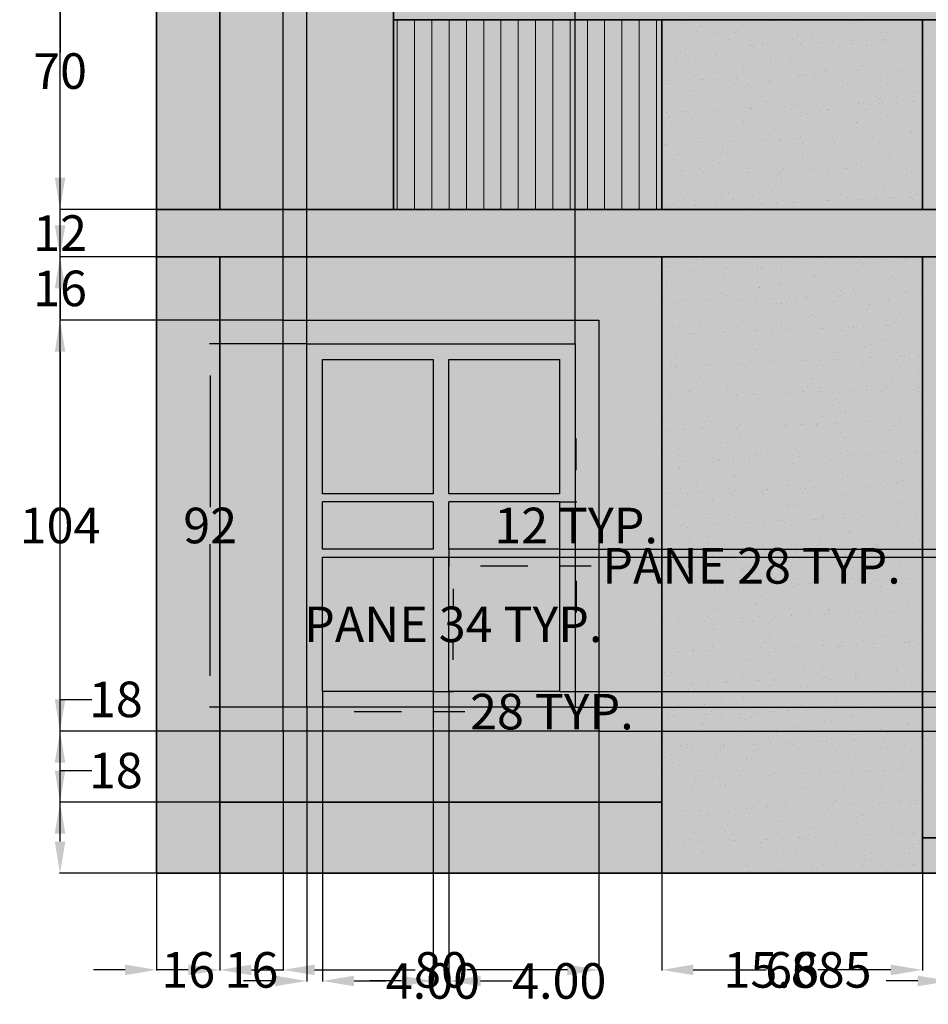
# Model space of a CAD drawing. Units: inches. Extents: x 207 to 609, y 30 to 576.
# Tile 1 of 4: x 215 to 445, y 30 to 279. Entities that reach past the tile are written whole.
import ezdxf

# ---------------------------------------------------------------- set-up
doc = ezdxf.new("R2010")
doc.units = ezdxf.units.IN
doc.header["$MEASUREMENT"] = 0
doc.layers.get('0').update_dxf_attribs({"color": 250})
for name, color, linetype, lineweight in [('A-ANNO-DIMS', 2, 'Continuous', 18), ('A-ELEV', 7, 'Continuous', 35), ('A-ELEV-PATT', 251, 'Continuous', 13), ('A-ELEV-PATT-CLAD', 67, 'Continuous', 13), ('A-ELEV-PATT-WOOD', 19, 'Continuous', 13), ('A-GLAZ', 4, 'Continuous', 25)]:
    doc.layers.add(name, color=color, linetype=linetype, lineweight=lineweight)
doc.styles.get("Standard").update_dxf_attribs({"font": 'arial.ttf'})
doc.dimstyles.get("Standard").update_dxf_attribs({"dimtxt": 9, "dimasz": 8, "dimexe": 0.18, "dimexo": 0.0625, "dimgap": 0.09, "dimtad": 0, "dimtih": 1, "dimtoh": 1, "dimdec": 0, "dimzin": 0, "dimdsep": 46, "dimlunit": 3, "dimtxsty": 'Standard', "dimcen": 0.09, "dimadec": 0, "dimazin": 0, "dimtfac": 1, "dimtdec": 0, "dimtofl": 0, "dimtmove": 0, "dimatfit": 3, "dimfxl": 1, "dimtolj": 1, "dimtzin": 0, "dimarcsym": 0})

# ---------------------------------------------------------------- blocks, each defined once
blk = doc.blocks.new('WIN-PANE-LG')
for p, q in [((0, 34), (28, 34)), ((0, 0), (0, 34)), ((28, 34), (28, 0)), ((28, 0), (0, 0))]:
    blk.add_line(p, q)
blk = doc.blocks.new('WIN-PANE-SM')
for p, q in [((28, 12), (0, 12)), ((0, 0), (0, 12)), ((28, 12), (28, 0)), ((28, 0), (0, 0))]:
    blk.add_line(p, q)
blk = doc.blocks.new('*D3')
at = {"layer": 'A-ANNO-DIMS', "color": 0, "lineweight": -2, "transparency": 16777216}
for p, q in [((319.76, 142.79), (324.98, 142.79)), ((324.8, 134.79), (324.8, 130.47)), ((324.8, 116.79), (324.8, 121.1)), ((319.76, 108.79), (324.98, 108.79))]:
    blk.add_line(p, q, dxfattribs=at)
at = {"layer": 'A-ANNO-DIMS', "color": 0, "transparency": 16777216}
for points in [[(323.46, 134.79), (326.13, 134.79), (324.8, 142.79)], [(323.46, 116.79), (326.13, 116.79), (324.8, 108.79)]]:
    blk.add_solid(points, dxfattribs=at)
at = {"layer": 'Defpoints', "color": 0, "transparency": 16777216}
for p in [(319.7, 142.79), (324.8, 142.79), (319.7, 108.79)]:
    blk.add_point(p, dxfattribs=at)
at = {"layer": 'A-ANNO-DIMS', "color": 0, "transparency": 16777216, "insert": (324.8, 125.79), "char_height": 9, "attachment_point": 5}
blk.add_mtext('\\A1;PANE 34 TYP.', dxfattribs=at)
blk = doc.blocks.new('*D4')
at = {"layer": 'A-ANNO-DIMS', "color": 0, "lineweight": -2, "transparency": 16777216}
for p, q in [((291.7, 108.72), (291.7, 103.51)), ((319.7, 108.72), (319.7, 103.51)), ((299.7, 103.69), (311.7, 103.69)), ((319.7, 103.69), (327.7, 103.69))]:
    blk.add_line(p, q, dxfattribs=at)
at = {"layer": 'A-ANNO-DIMS', "color": 0, "transparency": 16777216}
for points in [[(299.7, 105.02), (299.7, 102.35), (291.7, 103.69)], [(311.7, 105.02), (311.7, 102.35), (319.7, 103.69)]]:
    blk.add_solid(points, dxfattribs=at)
at = {"layer": 'Defpoints', "color": 0, "transparency": 16777216}
for p in [(291.7, 108.79), (319.7, 108.79), (319.7, 103.69)]:
    blk.add_point(p, dxfattribs=at)
at = {"layer": 'A-ANNO-DIMS', "color": 0, "transparency": 16777216, "insert": (349.77, 103.69), "char_height": 9, "attachment_point": 5}
blk.add_mtext('\\A1;28 TYP.', dxfattribs=at)
blk = doc.blocks.new('*D5')
at = {"layer": 'A-ANNO-DIMS', "color": 0, "lineweight": -2, "transparency": 16777216}
for p, q in [((323.7, 144.72), (323.7, 140.41)), ((351.7, 144.72), (351.7, 140.41)), ((331.7, 140.59), (343.7, 140.59)), ((351.7, 140.59), (359.7, 140.59))]:
    blk.add_line(p, q, dxfattribs=at)
at = {"layer": 'A-ANNO-DIMS', "color": 0, "transparency": 16777216}
for points in [[(331.7, 141.92), (331.7, 139.25), (323.7, 140.59)], [(343.7, 141.92), (343.7, 139.25), (351.7, 140.59)]]:
    blk.add_solid(points, dxfattribs=at)
at = {"layer": 'Defpoints', "color": 0, "transparency": 16777216}
for p in [(323.7, 144.79), (351.7, 144.79), (351.7, 140.59)]:
    blk.add_point(p, dxfattribs=at)
at = {"layer": 'A-ANNO-DIMS', "color": 0, "transparency": 16777216, "insert": (400.33, 140.59), "char_height": 9, "attachment_point": 5}
blk.add_mtext('\\A1;PANE 28 TYP.', dxfattribs=at)
blk = doc.blocks.new('*D6')
at = {"layer": 'A-ANNO-DIMS', "color": 0, "lineweight": -2, "transparency": 16777216}
for p, q in [((355.9, 164.79), (355.9, 172.79)), ((351.76, 156.79), (356.08, 156.79)), ((351.76, 144.79), (356.08, 144.79)), ((355.9, 136.79), (355.9, 128.79))]:
    blk.add_line(p, q, dxfattribs=at)
at = {"layer": 'A-ANNO-DIMS', "color": 0, "transparency": 16777216}
for points in [[(354.56, 164.79), (357.23, 164.79), (355.9, 156.79)], [(354.56, 136.79), (357.23, 136.79), (355.9, 144.79)]]:
    blk.add_solid(points, dxfattribs=at)
at = {"layer": 'Defpoints', "color": 0, "transparency": 16777216}
for p in [(351.7, 156.79), (355.9, 156.79), (351.7, 144.79)]:
    blk.add_point(p, dxfattribs=at)
at = {"layer": 'A-ANNO-DIMS', "color": 0, "transparency": 16777216, "insert": (355.9, 150.79), "char_height": 9, "attachment_point": 5}
blk.add_mtext('\\A1;12 TYP.', dxfattribs=at)
blk = doc.blocks.new('*D8')
at = {"layer": 'A-ANNO-DIMS', "color": 0, "lineweight": -2, "transparency": 16777216}
for p, q in [((249.63, 542.79), (225.07, 542.79)), ((225.25, 534.79), (225.25, 307.47)), ((225.25, 70.79), (225.25, 298.1)), ((249.63, 62.79), (225.07, 62.79))]:
    blk.add_line(p, q, dxfattribs=at)
at = {"layer": 'A-ANNO-DIMS', "color": 0, "transparency": 16777216}
for points in [[(223.91, 534.79), (226.58, 534.79), (225.25, 542.79)], [(223.91, 70.79), (226.58, 70.79), (225.25, 62.79)]]:
    blk.add_solid(points, dxfattribs=at)
at = {"layer": 'Defpoints', "color": 0, "transparency": 16777216}
for p in [(225.25, 542.79), (249.7, 542.79), (249.7, 62.79)]:
    blk.add_point(p, dxfattribs=at)
at = {"layer": 'A-ANNO-DIMS', "color": 0, "transparency": 16777216, "insert": (225.25, 302.79), "char_height": 9, "attachment_point": 5}
blk.add_mtext('\\A1;480', dxfattribs=at)
blk = doc.blocks.new('*D10')
at = {"layer": 'A-ANNO-DIMS', "color": 0, "lineweight": -2, "transparency": 16777216}
for p, q in [((225.25, 80.79), (225.25, 88.79)), ((225.25, 88.79), (233.25, 88.79)), ((265.63, 80.79), (225.07, 80.79)), ((225.25, 70.79), (225.25, 72.79)), ((265.63, 62.79), (225.07, 62.79))]:
    blk.add_line(p, q, dxfattribs=at)
at = {"layer": 'A-ANNO-DIMS', "color": 0, "transparency": 16777216}
for points in [[(223.91, 72.79), (226.58, 72.79), (225.25, 80.79)], [(223.91, 70.79), (226.58, 70.79), (225.25, 62.79)]]:
    blk.add_solid(points, dxfattribs=at)
at = {"layer": 'Defpoints', "color": 0, "transparency": 16777216}
for p in [(225.25, 80.79), (265.7, 80.79), (265.7, 62.79)]:
    blk.add_point(p, dxfattribs=at)
at = {"layer": 'A-ANNO-DIMS', "color": 0, "transparency": 16777216, "insert": (239.37, 88.79), "char_height": 9, "attachment_point": 5}
blk.add_mtext('\\A1;18', dxfattribs=at)
blk = doc.blocks.new('*D11')
at = {"layer": 'A-ANNO-DIMS', "color": 0, "lineweight": -2, "transparency": 16777216}
for p, q in [((225.25, 98.79), (225.25, 106.79)), ((225.25, 106.79), (233.25, 106.79)), ((281.63, 98.79), (225.07, 98.79)), ((225.25, 88.79), (225.25, 90.79)), ((265.63, 80.79), (225.07, 80.79))]:
    blk.add_line(p, q, dxfattribs=at)
at = {"layer": 'A-ANNO-DIMS', "color": 0, "transparency": 16777216}
for points in [[(223.91, 90.79), (226.58, 90.79), (225.25, 98.79)], [(223.91, 88.79), (226.58, 88.79), (225.25, 80.79)]]:
    blk.add_solid(points, dxfattribs=at)
at = {"layer": 'Defpoints', "color": 0, "transparency": 16777216}
for p in [(225.25, 98.79), (281.7, 98.79), (265.7, 80.79)]:
    blk.add_point(p, dxfattribs=at)
at = {"layer": 'A-ANNO-DIMS', "color": 0, "transparency": 16777216, "insert": (239.37, 106.79), "char_height": 9, "attachment_point": 5}
blk.add_mtext('\\A1;18', dxfattribs=at)
blk = doc.blocks.new('*D12')
at = {"layer": 'A-ANNO-DIMS', "color": 0, "lineweight": -2, "transparency": 16777216}
for p, q in [((281.63, 202.79), (225.07, 202.79)), ((225.25, 194.79), (225.25, 155.47)), ((225.25, 106.79), (225.25, 146.1)), ((281.63, 98.79), (225.07, 98.79))]:
    blk.add_line(p, q, dxfattribs=at)
at = {"layer": 'A-ANNO-DIMS', "color": 0, "transparency": 16777216}
for points in [[(223.91, 194.79), (226.58, 194.79), (225.25, 202.79)], [(223.91, 106.79), (226.58, 106.79), (225.25, 98.79)]]:
    blk.add_solid(points, dxfattribs=at)
at = {"layer": 'Defpoints', "color": 0, "transparency": 16777216}
for p in [(225.25, 202.79), (281.7, 202.79), (281.7, 98.79)]:
    blk.add_point(p, dxfattribs=at)
at = {"layer": 'A-ANNO-DIMS', "color": 0, "transparency": 16777216, "insert": (225.25, 150.79), "char_height": 9, "attachment_point": 5}
blk.add_mtext('\\A1;104', dxfattribs=at)
blk = doc.blocks.new('*D13')
at = {"layer": 'A-ANNO-DIMS', "color": 0, "lineweight": -2, "transparency": 16777216}
for p, q in [((225.25, 226.79), (225.25, 234.79)), ((265.63, 218.79), (225.07, 218.79)), ((281.63, 202.79), (225.07, 202.79)), ((225.25, 194.79), (225.25, 186.79))]:
    blk.add_line(p, q, dxfattribs=at)
at = {"layer": 'A-ANNO-DIMS', "color": 0, "transparency": 16777216}
for points in [[(223.91, 226.79), (226.58, 226.79), (225.25, 218.79)], [(223.91, 194.79), (226.58, 194.79), (225.25, 202.79)]]:
    blk.add_solid(points, dxfattribs=at)
at = {"layer": 'Defpoints', "color": 0, "transparency": 16777216}
for p in [(225.25, 218.79), (265.7, 218.79), (281.7, 202.79)]:
    blk.add_point(p, dxfattribs=at)
at = {"layer": 'A-ANNO-DIMS', "color": 0, "transparency": 16777216, "insert": (225.25, 210.79), "char_height": 9, "attachment_point": 5}
blk.add_mtext('\\A1;16', dxfattribs=at)
blk = doc.blocks.new('*D14')
at = {"layer": 'A-ANNO-DIMS', "color": 0, "lineweight": -2, "transparency": 16777216}
for p, q in [((225.25, 238.79), (225.25, 246.79)), ((265.63, 230.79), (225.07, 230.79)), ((265.63, 218.79), (225.07, 218.79)), ((225.25, 210.79), (225.25, 202.79))]:
    blk.add_line(p, q, dxfattribs=at)
at = {"layer": 'A-ANNO-DIMS', "color": 0, "transparency": 16777216}
for points in [[(223.91, 238.79), (226.58, 238.79), (225.25, 230.79)], [(223.91, 210.79), (226.58, 210.79), (225.25, 218.79)]]:
    blk.add_solid(points, dxfattribs=at)
at = {"layer": 'Defpoints', "color": 0, "transparency": 16777216}
for p in [(225.25, 230.79), (265.7, 230.79), (265.7, 218.79)]:
    blk.add_point(p, dxfattribs=at)
at = {"layer": 'A-ANNO-DIMS', "color": 0, "transparency": 16777216, "insert": (225.25, 224.79), "char_height": 9, "attachment_point": 5}
blk.add_mtext('\\A1;12', dxfattribs=at)
blk = doc.blocks.new('*D15')
at = {"layer": 'A-ANNO-DIMS', "color": 0, "lineweight": -2, "transparency": 16777216}
for p, q in [((265.63, 300.79), (225.07, 300.79)), ((225.25, 292.79), (225.25, 270.47)), ((225.25, 238.79), (225.25, 261.1)), ((265.63, 230.79), (225.07, 230.79))]:
    blk.add_line(p, q, dxfattribs=at)
at = {"layer": 'A-ANNO-DIMS', "color": 0, "transparency": 16777216}
for points in [[(223.91, 292.79), (226.58, 292.79), (225.25, 300.79)], [(223.91, 238.79), (226.58, 238.79), (225.25, 230.79)]]:
    blk.add_solid(points, dxfattribs=at)
at = {"layer": 'Defpoints', "color": 0, "transparency": 16777216}
for p in [(225.25, 300.79), (265.7, 300.79), (265.7, 230.79)]:
    blk.add_point(p, dxfattribs=at)
at = {"layer": 'A-ANNO-DIMS', "color": 0, "transparency": 16777216, "insert": (225.25, 265.79), "char_height": 9, "attachment_point": 5}
blk.add_mtext('\\A1;70', dxfattribs=at)
blk = doc.blocks.new('*D27')
at = {"layer": 'A-ANNO-DIMS', "color": 0, "lineweight": -2, "transparency": 16777216}
for p, q in [((249.7, 62.72), (249.7, 38.16)), ((265.7, 62.72), (265.7, 38.16)), ((241.7, 38.34), (233.7, 38.34)), ((273.7, 38.34), (281.7, 38.34))]:
    blk.add_line(p, q, dxfattribs=at)
at = {"layer": 'A-ANNO-DIMS', "color": 0, "transparency": 16777216}
for points in [[(241.7, 39.67), (241.7, 37), (249.7, 38.34)], [(273.7, 39.67), (273.7, 37), (265.7, 38.34)]]:
    blk.add_solid(points, dxfattribs=at)
at = {"layer": 'Defpoints', "color": 0, "transparency": 16777216}
for p in [(249.7, 62.79), (265.7, 62.79), (265.7, 38.34)]:
    blk.add_point(p, dxfattribs=at)
at = {"layer": 'A-ANNO-DIMS', "color": 0, "transparency": 16777216, "insert": (257.7, 38.34), "char_height": 9, "attachment_point": 5}
blk.add_mtext('\\A1;16', dxfattribs=at)
blk = doc.blocks.new('*D28')
at = {"layer": 'A-ANNO-DIMS', "color": 0, "lineweight": -2, "transparency": 16777216}
for p, q in [((281.7, 98.72), (281.7, 38.16)), ((265.7, 62.72), (265.7, 38.16)), ((257.7, 38.34), (249.7, 38.34)), ((289.7, 38.34), (297.7, 38.34))]:
    blk.add_line(p, q, dxfattribs=at)
at = {"layer": 'A-ANNO-DIMS', "color": 0, "transparency": 16777216}
for points in [[(257.7, 39.67), (257.7, 37), (265.7, 38.34)], [(289.7, 39.67), (289.7, 37), (281.7, 38.34)]]:
    blk.add_solid(points, dxfattribs=at)
at = {"layer": 'Defpoints', "color": 0, "transparency": 16777216}
for p in [(281.7, 98.79), (265.7, 62.79), (281.7, 38.34)]:
    blk.add_point(p, dxfattribs=at)
at = {"layer": 'A-ANNO-DIMS', "color": 0, "transparency": 16777216, "insert": (273.7, 38.34), "char_height": 9, "attachment_point": 5}
blk.add_mtext('\\A1;16', dxfattribs=at)
blk = doc.blocks.new('*D29')
at = {"layer": 'A-ANNO-DIMS', "color": 0, "lineweight": -2, "transparency": 16777216}
for p, q in [((281.7, 98.72), (281.7, 38.16)), ((361.7, 98.72), (361.7, 38.16)), ((289.7, 38.34), (315.17, 38.34)), ((353.7, 38.34), (328.22, 38.34))]:
    blk.add_line(p, q, dxfattribs=at)
at = {"layer": 'A-ANNO-DIMS', "color": 0, "transparency": 16777216}
for points in [[(289.7, 39.67), (289.7, 37), (281.7, 38.34)], [(353.7, 39.67), (353.7, 37), (361.7, 38.34)]]:
    blk.add_solid(points, dxfattribs=at)
at = {"layer": 'Defpoints', "color": 0, "transparency": 16777216}
for p in [(281.7, 98.79), (361.7, 98.79), (361.7, 38.34)]:
    blk.add_point(p, dxfattribs=at)
at = {"layer": 'A-ANNO-DIMS', "color": 0, "transparency": 16777216, "insert": (321.7, 38.34), "char_height": 9, "attachment_point": 5}
blk.add_mtext('\\A1;80', dxfattribs=at)
blk = doc.blocks.new('*D30')
at = {"layer": 'A-ANNO-DIMS', "color": 0, "lineweight": -2, "transparency": 16777216}
for p, q in [((361.7, 98.72), (361.7, 38.16)), ((377.58, 62.72), (377.58, 38.16)), ((353.7, 38.34), (345.7, 38.34)), ((385.58, 38.34), (393.58, 38.34))]:
    blk.add_line(p, q, dxfattribs=at)
at = {"layer": 'A-ANNO-DIMS', "color": 0, "transparency": 16777216}
for points in [[(353.7, 39.67), (353.7, 37), (361.7, 38.34)], [(385.58, 39.67), (385.58, 37), (377.58, 38.34)]]:
    blk.add_solid(points, dxfattribs=at)
at = {"layer": 'Defpoints', "color": 0, "transparency": 16777216}
for p in [(361.7, 98.79), (377.58, 62.79), (377.58, 38.34)]:
    blk.add_point(p, dxfattribs=at)
at = {"layer": 'A-ANNO-DIMS', "color": 0, "transparency": 16777216, "insert": (411.96, 38.34), "char_height": 9, "attachment_point": 5}
blk.add_mtext('\\A1;15.885', dxfattribs=at)
blk = doc.blocks.new('*D31')
at = {"layer": 'A-ANNO-DIMS', "color": 0, "lineweight": -2, "transparency": 16777216}
for p, q in [((377.58, 62.72), (377.58, 38.16)), ((443.58, 62.72), (443.58, 38.16)), ((385.58, 38.34), (404.02, 38.34)), ((435.58, 38.34), (417.14, 38.34))]:
    blk.add_line(p, q, dxfattribs=at)
at = {"layer": 'A-ANNO-DIMS', "color": 0, "transparency": 16777216}
for points in [[(385.58, 39.67), (385.58, 37), (377.58, 38.34)], [(435.58, 39.67), (435.58, 37), (443.58, 38.34)]]:
    blk.add_solid(points, dxfattribs=at)
at = {"layer": 'Defpoints', "color": 0, "transparency": 16777216}
for p in [(377.58, 62.79), (443.58, 62.79), (443.58, 38.34)]:
    blk.add_point(p, dxfattribs=at)
at = {"layer": 'A-ANNO-DIMS', "color": 0, "transparency": 16777216, "insert": (410.58, 38.34), "char_height": 9, "attachment_point": 5}
blk.add_mtext('\\A1;66', dxfattribs=at)
blk = doc.blocks.new('*D32')
at = {"layer": 'A-ANNO-DIMS', "color": 0, "lineweight": -2, "transparency": 16777216}
for p, q in [((450.42, 269.6), (450.42, 38.16)), ((443.58, 62.72), (443.58, 38.16)), ((435.58, 38.34), (427.58, 38.34)), ((458.42, 38.34), (466.42, 38.34))]:
    blk.add_line(p, q, dxfattribs=at)
at = {"layer": 'A-ANNO-DIMS', "color": 0, "transparency": 16777216}
for points in [[(435.58, 39.67), (435.58, 37), (443.58, 38.34)], [(458.42, 39.67), (458.42, 37), (450.42, 38.34)]]:
    blk.add_solid(points, dxfattribs=at)
at = {"layer": 'Defpoints', "color": 0, "transparency": 16777216}
for p in [(450.42, 269.66), (443.58, 62.79), (450.42, 38.34)]:
    blk.add_point(p, dxfattribs=at)
at = {"layer": 'A-ANNO-DIMS', "color": 0, "transparency": 16777216, "insert": (481.71, 38.34), "char_height": 9, "attachment_point": 5}
blk.add_mtext('\\A1;6.844', dxfattribs=at)
blk = doc.blocks.new('*D61')
at = {"layer": 'A-ANNO-DIMS', "color": 0, "lineweight": -2, "transparency": 16777216}
for p, q in [((287.63, 196.79), (263.07, 196.79)), ((263.25, 188.79), (263.25, 155.47)), ((263.25, 112.79), (263.25, 146.1)), ((287.63, 104.79), (263.07, 104.79))]:
    blk.add_line(p, q, dxfattribs=at)
at = {"layer": 'A-ANNO-DIMS', "color": 0, "transparency": 16777216}
for points in [[(261.91, 188.79), (264.58, 188.79), (263.25, 196.79)], [(261.91, 112.79), (264.58, 112.79), (263.25, 104.79)]]:
    blk.add_solid(points, dxfattribs=at)
at = {"layer": 'Defpoints', "color": 0, "transparency": 16777216}
for p in [(263.25, 196.79), (287.7, 196.79), (287.7, 104.79)]:
    blk.add_point(p, dxfattribs=at)
at = {"layer": 'A-ANNO-DIMS', "color": 0, "transparency": 16777216, "insert": (263.25, 150.79), "char_height": 9, "attachment_point": 5}
blk.add_mtext('\\A1;92', dxfattribs=at)
blk = doc.blocks.new('*D71')
at = {"layer": 'A-ANNO-DIMS', "color": 0, "lineweight": -2, "transparency": 16777216}
for p, q in [((273.7, 570.04), (265.7, 570.04)), ((281.7, 202.85), (281.7, 570.22)), ((287.7, 196.85), (287.7, 570.22)), ((295.7, 570.04), (303.7, 570.04))]:
    blk.add_line(p, q, dxfattribs=at)
at = {"layer": 'A-ANNO-DIMS', "color": 0, "transparency": 16777216}
for points in [[(273.7, 571.37), (273.7, 568.7), (281.7, 570.04)], [(295.7, 571.37), (295.7, 568.7), (287.7, 570.04)]]:
    blk.add_solid(points, dxfattribs=at)
at = {"layer": 'Defpoints', "color": 0, "transparency": 16777216}
for p in [(287.7, 570.04), (281.7, 202.79), (287.7, 196.79)]:
    blk.add_point(p, dxfattribs=at)
at = {"layer": 'A-ANNO-DIMS', "color": 0, "transparency": 16777216, "insert": (315.48, 570.04), "char_height": 9, "attachment_point": 5}
blk.add_mtext('\\A1;6.00', dxfattribs=at)
blk = doc.blocks.new('*D72')
at = {"layer": 'A-ANNO-DIMS', "color": 0, "lineweight": -2, "transparency": 16777216}
for p, q in [((287.7, 196.85), (287.7, 570.22)), ((295.7, 570.04), (306.41, 570.04)), ((347.7, 570.04), (336.98, 570.04)), ((355.7, 196.85), (355.7, 570.22))]:
    blk.add_line(p, q, dxfattribs=at)
at = {"layer": 'A-ANNO-DIMS', "color": 0, "transparency": 16777216}
for points in [[(295.7, 571.37), (295.7, 568.7), (287.7, 570.04)], [(347.7, 571.37), (347.7, 568.7), (355.7, 570.04)]]:
    blk.add_solid(points, dxfattribs=at)
at = {"layer": 'Defpoints', "color": 0, "transparency": 16777216}
for p in [(355.7, 570.04), (287.7, 196.79), (355.7, 196.79)]:
    blk.add_point(p, dxfattribs=at)
at = {"layer": 'A-ANNO-DIMS', "color": 0, "transparency": 16777216, "insert": (321.7, 570.04), "char_height": 9, "attachment_point": 5}
blk.add_mtext('\\A1;68.00', dxfattribs=at)
blk = doc.blocks.new('*D73')
at = {"layer": 'A-ANNO-DIMS', "color": 0, "lineweight": -2, "transparency": 16777216}
for p, q in [((291.7, 108.72), (291.7, 35.36)), ((287.7, 104.72), (287.7, 35.36)), ((279.7, 35.54), (271.7, 35.54)), ((299.7, 35.54), (307.7, 35.54))]:
    blk.add_line(p, q, dxfattribs=at)
at = {"layer": 'A-ANNO-DIMS', "color": 0, "transparency": 16777216}
for points in [[(279.7, 36.87), (279.7, 34.2), (287.7, 35.54)], [(299.7, 36.87), (299.7, 34.2), (291.7, 35.54)]]:
    blk.add_solid(points, dxfattribs=at)
at = {"layer": 'Defpoints', "color": 0, "transparency": 16777216}
for p in [(291.7, 108.79), (287.7, 104.79), (291.7, 35.54)]:
    blk.add_point(p, dxfattribs=at)
at = {"layer": 'A-ANNO-DIMS', "color": 0, "transparency": 16777216, "insert": (319.64, 35.54), "char_height": 9, "attachment_point": 5}
blk.add_mtext('\\A1;4.00', dxfattribs=at)
blk = doc.blocks.new('*D74')
at = {"layer": 'A-ANNO-DIMS', "color": 0, "lineweight": -2, "transparency": 16777216}
for p, q in [((319.7, 108.72), (319.7, 35.36)), ((323.7, 108.72), (323.7, 35.36)), ((311.7, 35.54), (303.7, 35.54)), ((331.7, 35.54), (339.7, 35.54))]:
    blk.add_line(p, q, dxfattribs=at)
at = {"layer": 'A-ANNO-DIMS', "color": 0, "transparency": 16777216}
for points in [[(311.7, 36.87), (311.7, 34.2), (319.7, 35.54)], [(331.7, 36.87), (331.7, 34.2), (323.7, 35.54)]]:
    blk.add_solid(points, dxfattribs=at)
at = {"layer": 'Defpoints', "color": 0, "transparency": 16777216}
for p in [(319.7, 108.79), (323.7, 108.79), (323.7, 35.54)]:
    blk.add_point(p, dxfattribs=at)
at = {"layer": 'A-ANNO-DIMS', "color": 0, "transparency": 16777216, "insert": (351.64, 35.54), "char_height": 9, "attachment_point": 5}
blk.add_mtext('\\A1;4.00', dxfattribs=at)
blk = doc.blocks.new('*D75')
at = {"layer": 'A-ANNO-DIMS', "color": 0, "lineweight": -2, "transparency": 16777216}
for p, q in [((576.95, 112.79), (576.95, 120.79)), ((576.95, 120.79), (584.95, 120.79)), ((355.76, 104.79), (577.13, 104.79)), ((361.76, 98.79), (577.13, 98.79)), ((576.95, 90.79), (576.95, 82.79))]:
    blk.add_line(p, q, dxfattribs=at)
at = {"layer": 'A-ANNO-DIMS', "color": 0, "transparency": 16777216}
for points in [[(575.61, 112.79), (578.28, 112.79), (576.95, 104.79)], [(575.61, 90.79), (578.28, 90.79), (576.95, 98.79)]]:
    blk.add_solid(points, dxfattribs=at)
at = {"layer": 'Defpoints', "color": 0, "transparency": 16777216}
for p in [(355.7, 104.79), (576.95, 104.79), (361.7, 98.79)]:
    blk.add_point(p, dxfattribs=at)
at = {"layer": 'A-ANNO-DIMS', "color": 0, "transparency": 16777216, "insert": (596.73, 120.79), "char_height": 9, "attachment_point": 5}
blk.add_mtext('\\A1;6.00', dxfattribs=at)
blk = doc.blocks.new('*D76')
at = {"layer": 'A-ANNO-DIMS', "color": 0, "lineweight": -2, "transparency": 16777216}
for p, q in [((576.95, 116.79), (576.95, 124.79)), ((576.95, 124.79), (584.95, 124.79)), ((351.76, 108.79), (577.13, 108.79)), ((355.76, 104.79), (577.13, 104.79)), ((576.95, 96.79), (576.95, 88.79))]:
    blk.add_line(p, q, dxfattribs=at)
at = {"layer": 'A-ANNO-DIMS', "color": 0, "transparency": 16777216}
for points in [[(575.61, 116.79), (578.28, 116.79), (576.95, 108.79)], [(575.61, 96.79), (578.28, 96.79), (576.95, 104.79)]]:
    blk.add_solid(points, dxfattribs=at)
at = {"layer": 'Defpoints', "color": 0, "transparency": 16777216}
for p in [(351.7, 108.79), (576.95, 108.79), (355.7, 104.79)]:
    blk.add_point(p, dxfattribs=at)
at = {"layer": 'A-ANNO-DIMS', "color": 0, "transparency": 16777216, "insert": (596.89, 124.79), "char_height": 9, "attachment_point": 5}
blk.add_mtext('\\A1;4.00', dxfattribs=at)
blk = doc.blocks.new('*D77')
at = {"layer": 'A-ANNO-DIMS', "color": 0, "lineweight": -2, "transparency": 16777216}
for p, q in [((576.95, 152.79), (576.95, 160.79)), ((576.95, 160.79), (584.95, 160.79)), ((351.76, 144.79), (577.13, 144.79)), ((351.76, 142.79), (577.13, 142.79)), ((576.95, 134.79), (576.95, 126.79))]:
    blk.add_line(p, q, dxfattribs=at)
at = {"layer": 'A-ANNO-DIMS', "color": 0, "transparency": 16777216}
for points in [[(575.61, 152.79), (578.28, 152.79), (576.95, 144.79)], [(575.61, 134.79), (578.28, 134.79), (576.95, 142.79)]]:
    blk.add_solid(points, dxfattribs=at)
at = {"layer": 'Defpoints', "color": 0, "transparency": 16777216}
for p in [(351.7, 144.79), (576.95, 144.79), (351.7, 142.79)]:
    blk.add_point(p, dxfattribs=at)
at = {"layer": 'A-ANNO-DIMS', "color": 0, "transparency": 16777216, "insert": (596.79, 160.79), "char_height": 9, "attachment_point": 5}
blk.add_mtext('\\A1;2.00', dxfattribs=at)
blk = doc.blocks.new('*D79')
at = {"layer": 'A-ANNO-DIMS', "color": 0, "lineweight": -2, "transparency": 16777216}
for p, q in [((453.42, 240.19), (453.42, 35.36)), ((450.42, 237.19), (450.42, 35.36)), ((442.42, 35.54), (434.42, 35.54)), ((461.42, 35.54), (469.42, 35.54))]:
    blk.add_line(p, q, dxfattribs=at)
at = {"layer": 'A-ANNO-DIMS', "color": 0, "transparency": 16777216}
for points in [[(442.42, 36.87), (442.42, 34.2), (450.42, 35.54)], [(461.42, 36.87), (461.42, 34.2), (453.42, 35.54)]]:
    blk.add_solid(points, dxfattribs=at)
at = {"layer": 'Defpoints', "color": 0, "transparency": 16777216}
for p in [(453.42, 240.26), (450.42, 237.26), (453.42, 35.54)]:
    blk.add_point(p, dxfattribs=at)
at = {"layer": 'A-ANNO-DIMS', "color": 0, "transparency": 16777216, "insert": (481.19, 35.54), "char_height": 9, "attachment_point": 5}
blk.add_mtext('\\A1;3.00', dxfattribs=at)

msp = doc.modelspace()

# ---------------------------------------------------------------- hatches: boundary and pattern name
at = {"layer": 'A-ELEV-PATT'}
h = msp.add_hatch(color=256, dxfattribs=at)
h.dxf.hatch_style = 1
h.paths.add_polyline_path([(549.6956, 542.7864), (443.656, 542.7864), (443.656, 470.7864), (549.6956, 470.7864)])
h.paths.add_polyline_path([(549.6956, 230.7864), (249.6956, 230.7864), (249.6956, 218.7864), (549.6956, 218.7864)])
h.paths.add_polyline_path([(377.5808, 80.7864), (265.6956, 80.7864), (265.6956, 62.7864), (377.5808, 62.7864)])
h.paths.add_polyline_path([(549.6956, 71.7864), (443.5808, 71.7864), (443.5808, 62.7864), (549.6956, 62.7864)])
h = msp.add_hatch(color=256, dxfattribs=at)
h.dxf.hatch_style = 1
h.paths.add_polyline_path([(549.6956, 470.7864), (309.6956, 470.7864), (309.6956, 278.7864), (549.6956, 278.7864), (549.6956, 302.7864), (324.6956, 302.7864), (324.6956, 455.7864), (549.6956, 455.7864)])
h = msp.add_hatch(color=256, dxfattribs=at)
h.dxf.hatch_style = 1
h.paths.add_polyline_path([(265.6956, 302.7864), (249.6956, 302.7864), (249.6956, 230.7864), (265.6956, 230.7864)])
h.paths.add_polyline_path([(265.6956, 218.7864), (249.6956, 218.7864), (249.6956, 62.7864), (265.6956, 62.7864)])
h.paths.add_polyline_path([(549.6956, 278.7864), (443.5808, 278.7864), (443.5808, 230.7864), (549.6956, 230.7864)])
h.paths.add_polyline_path([(534.6005, 237.2568), (450.425, 237.2568), (450.425, 269.6636), (534.6005, 269.6636)], flags=16)
h.paths.add_polyline_path([(531.6005, 240.2568), (453.425, 240.2568), (453.425, 266.6636), (531.6005, 266.6636)], flags=0)
at = {"layer": 'A-ELEV-PATT', "transparency": 33554656}
h = msp.add_hatch(color=256, dxfattribs=at)
h.set_gradient(color1=(215, 235, 210), color2=(99, 100, 102), rotation=180)
h.paths.add_polyline_path([(265.6956, 230.7864), (309.6956, 230.7864), (309.6956, 300.7864), (265.6956, 300.7864)])
h = msp.add_hatch(color=256, dxfattribs=at)
h.paths.add_polyline_path([(443.5808, 278.7864), (377.5808, 278.7864), (377.5808, 230.7864), (443.5808, 230.7864)])
h.paths.add_polyline_path([(443.5808, 218.7864), (377.5808, 218.7864), (377.5808, 62.7864), (443.5808, 62.7864)])
h = msp.add_hatch(dxfattribs=at)
h.set_pattern_fill('AR-SAND', color=256, scale=3, angle=45, style=0)
h.paths.add_polyline_path([(443.5808, 218.7864), (377.5808, 218.7864), (377.5808, 62.7864), (443.5808, 62.7864)])
h.paths.add_polyline_path([(443.5808, 278.7864), (377.5808, 278.7864), (377.5808, 230.7864), (443.5808, 230.7864)])
h = msp.add_hatch(color=256, dxfattribs=at)
h.paths.add_polyline_path([(377.5808, 218.7864), (265.6956, 218.7864), (265.6956, 80.7864), (377.5808, 80.7864)])
h.paths.add_polyline_path([(361.6956, 202.7864), (361.6956, 98.7864), (281.6956, 98.7864), (281.6956, 202.7864)], flags=16)
h.paths.add_polyline_path([(355.6956, 196.7864), (355.6956, 104.7864), (287.6956, 104.7864), (287.6956, 196.7864)], flags=0)
h.paths.add_polyline_path([(351.6956, 192.7864), (351.6956, 158.7864), (323.6956, 158.7864), (323.6956, 192.7864)], flags=0)
h.paths.add_polyline_path([(319.6956, 192.7864), (319.6956, 158.7864), (291.6956, 158.7864), (291.6956, 192.7864)], flags=0)
h.paths.add_polyline_path([(351.6956, 156.7864), (351.6956, 144.7864), (323.6956, 144.7864), (323.6956, 156.7864)], flags=0)
h.paths.add_polyline_path([(319.6956, 156.7864), (319.6956, 144.7864), (291.6956, 144.7864), (291.6956, 156.7864)], flags=0)
h.paths.add_polyline_path([(351.6956, 142.7864), (351.6956, 108.7864), (323.6956, 108.7864), (323.6956, 142.7864)], flags=0)
h.paths.add_polyline_path([(319.6956, 142.7864), (319.6956, 108.7864), (291.6956, 108.7864), (291.6956, 142.7864)], flags=0)
msp.add_hatch(color=256, dxfattribs=at).paths.add_polyline_path([(549.6956, 218.7864), (443.5808, 218.7864), (443.5808, 71.7864), (446.5808, 71.7864), (446.5808, 206.7864), (542.5808, 206.7864), (542.5808, 71.7864), (549.6956, 71.7864)])
h = msp.add_hatch(color=256, dxfattribs=at)
h.paths.add_polyline_path([(355.6956, 202.7864), (287.6956, 202.7864), (287.6956, 196.7864), (355.6956, 196.7864)])
h.paths.add_polyline_path([(361.6956, 196.7864), (355.6956, 196.7864), (355.6956, 104.7864), (361.6956, 104.7864)])
h.paths.add_polyline_path([(355.6956, 104.7864), (287.6956, 104.7864), (287.6956, 98.7864), (355.6956, 98.7864)])
h.paths.add_polyline_path([(287.6956, 104.7864), (281.6956, 104.7864), (281.6956, 98.7864), (287.6956, 98.7864)])
h.paths.add_polyline_path([(287.6956, 196.7864), (281.6956, 196.7864), (281.6956, 104.7864), (287.6956, 104.7864)])
h.paths.add_polyline_path([(287.6956, 202.7864), (281.6956, 202.7864), (281.6956, 196.7864), (287.6956, 196.7864)])
h.paths.add_polyline_path([(361.6956, 202.7864), (355.6956, 202.7864), (355.6956, 196.7864), (361.6956, 196.7864)])
h.paths.add_polyline_path([(361.6956, 104.7864), (355.6956, 104.7864), (355.6956, 98.7864), (361.6956, 98.7864)])
at = {"layer": 'A-ELEV-PATT-CLAD', "transparency": 33554656}
h = msp.add_hatch(dxfattribs=at)
h.set_pattern_fill('ANSI31', color=256, scale=35, angle=45, style=0)
h.paths.add_polyline_path([(377.5808, 278.7864), (309.6956, 278.7864), (309.6956, 230.7864), (377.5808, 230.7864)])
at = {"layer": 'A-ELEV-PATT-WOOD', "transparency": 33554656}
msp.add_hatch(color=256, dxfattribs=at).paths.add_polyline_path([(377.5808, 278.7864), (309.6956, 278.7864), (309.6956, 230.7864), (377.5808, 230.7864)])
h = msp.add_hatch(color=256, dxfattribs=at)
h.paths.add_polyline_path([(450.425, 269.6636), (450.425, 237.2568), (534.6005, 237.2568), (534.6005, 269.6636)])
h.paths.add_polyline_path([(531.6005, 266.6636), (531.6005, 240.2568), (453.425, 240.2568), (453.425, 266.6636)], flags=16)
h.paths.add_polyline_path([(446.5808, 206.7864), (446.5808, 71.7864), (542.5808, 71.7864), (542.5808, 206.7864)])
h.paths.add_polyline_path([(512.5808, 200.7864), (536.5808, 200.7864), (536.5808, 77.7864), (512.5808, 77.7864)], flags=16)
h.paths.add_polyline_path([(355.6956, 196.7864), (287.6956, 196.7864), (287.6956, 104.7864), (355.6956, 104.7864)])
h.paths.add_polyline_path([(319.6956, 192.7864), (319.6956, 158.7864), (291.6956, 158.7864), (291.6956, 192.7864)], flags=16)
h.paths.add_polyline_path([(323.6956, 192.7864), (351.6956, 192.7864), (351.6956, 158.7864), (323.6956, 158.7864)], flags=16)
h.paths.add_polyline_path([(319.6956, 156.7864), (319.6956, 144.7864), (291.6956, 144.7864), (291.6956, 156.7864)], flags=16)
h.paths.add_polyline_path([(323.6956, 156.7864), (351.6956, 156.7864), (351.6956, 144.7864), (323.6956, 144.7864)], flags=16)
h.paths.add_polyline_path([(319.6956, 142.7864), (319.6956, 108.7864), (291.6956, 108.7864), (291.6956, 142.7864)], flags=16)
h.paths.add_polyline_path([(323.6956, 142.7864), (351.6956, 142.7864), (351.6956, 108.7864), (323.6956, 108.7864)], flags=16)
h.paths.add_polyline_path([(496.5808, 139.2864), (497.5808, 139.2864), (497.5808, 151.2864), (496.5808, 151.2864)], flags=16)
h.paths.add_polyline_path([(490.5808, 151.2864), (489.5808, 151.2864), (489.5808, 139.2864), (490.5808, 139.2864)], flags=0)
h = msp.add_hatch(color=256, dxfattribs=at)
h.paths.add_polyline_path([(531.6005, 266.6636), (453.425, 266.6636), (453.425, 240.2568), (531.6005, 240.2568)])
h.paths.add_polyline_path([(351.6956, 192.7864), (323.6956, 192.7864), (323.6956, 158.7864), (351.6956, 158.7864)])
h.paths.add_polyline_path([(319.6956, 192.7864), (291.6956, 192.7864), (291.6956, 158.7864), (319.6956, 158.7864)])
h.paths.add_polyline_path([(319.6956, 156.7864), (291.6956, 156.7864), (291.6956, 144.7864), (319.6956, 144.7864)])
h.paths.add_polyline_path([(351.6956, 156.7864), (323.6956, 156.7864), (323.6956, 144.7864), (351.6956, 144.7864)])
h.paths.add_polyline_path([(351.6956, 142.7864), (323.6956, 142.7864), (323.6956, 108.7864), (351.6956, 108.7864)])
h.paths.add_polyline_path([(319.6956, 142.7864), (291.6956, 142.7864), (291.6956, 108.7864), (319.6956, 108.7864)])
h.paths.add_polyline_path([(536.5808, 200.7864), (512.5808, 200.7864), (512.5808, 77.7864), (536.5808, 77.7864)])

# ---------------------------------------------------------------- linework, layer by layer
at = {"layer": 'A-ELEV'}
for p, q in [((249.6956, 542.7864), (249.6956, 62.7864)), ((309.6956, 470.7864), (309.6956, 230.7864)), ((265.6956, 302.7864), (265.6956, 230.7864)), ((549.6956, 278.7864), (309.6956, 278.7864)), ((377.5808, 278.7864), (377.5808, 230.7864)), ((443.5808, 278.7864), (443.5808, 230.7864)), ((549.6956, 230.7864), (249.6956, 230.7864)), ((549.6956, 218.7864), (249.6956, 218.7864)), ((265.6956, 218.7864), (265.6956, 62.7864)), ((377.5808, 218.7864), (377.5808, 62.7864)), ((443.5808, 218.7864), (443.5808, 62.7864)), ((377.5808, 80.7864), (265.6956, 80.7864)), ((549.6956, 71.7864), (443.5808, 71.7864)), ((549.6956, 62.7864), (249.6956, 62.7864))]:
    msp.add_line(p, q, dxfattribs=at)
at = {"layer": 'A-GLAZ'}
for p, q in [((281.6956, 202.7864), (361.6956, 202.7864)), ((281.6956, 98.7864), (281.6956, 202.7864)), ((361.6956, 202.7864), (361.6956, 98.7864)), ((287.6956, 104.7864), (287.6956, 196.7864)), ((287.6956, 196.7864), (355.6956, 196.7864)), ((355.6956, 196.7864), (355.6956, 104.7864)), ((355.6956, 104.7864), (287.6956, 104.7864)), ((361.6956, 98.7864), (281.6956, 98.7864))]:
    msp.add_line(p, q, dxfattribs=at)

# ---------------------------------------------------------------- block references
for name, p in [('WIN-PANE-LG', (291.696, 158.786)), ('WIN-PANE-SM', (291.696, 144.786)), ('WIN-PANE-SM', (323.696, 144.786)), ('WIN-PANE-LG', (291.696, 108.786))]:
    msp.add_blockref(name, p, dxfattribs=at)
at = {"layer": 'A-GLAZ', "rotation": 180}
for p in [(351.6951, 192.7869), (351.6951, 142.7869)]:
    msp.add_blockref('WIN-PANE-LG', p, dxfattribs=at)

# ---------------------------------------------------------------- dimensions: what is measured, and where the dimension line sits
at = {"layer": 'A-ANNO-DIMS'}
for base, p1, p2, override, picture, middle in [((287.6956, 570.0364), (281.6956, 202.7864), (287.6956, 196.7864), {"dimdec": 2, "dimlfac": 1, "dimrnd": 0, "dimzin": 0, "dimdsep": 46, "dimlunit": 2}, '*D71', (315.4837, 570.0364)), ((355.6956, 570.0364), (287.6956, 196.7864), (355.6956, 196.7864), {"dimdec": 2, "dimlfac": 1, "dimrnd": 0, "dimzin": 0, "dimdsep": 46, "dimlunit": 2}, '*D72', (321.6956, 570.0364)), ((450.425, 38.3364), (443.5808, 62.7864), (450.425, 269.6636), {"dimdec": 3, "dimlfac": 1, "dimrnd": 0, "dimzin": 0, "dimdsep": 46, "dimlunit": 2}, '*D32', (481.7063, 38.3364)), ((453.425, 35.5364), (450.425, 237.2568), (453.425, 240.2568), {"dimdec": 2, "dimlfac": 1, "dimrnd": 0, "dimzin": 0, "dimdsep": 46, "dimlunit": 2}, '*D79', (481.1855, 35.5364)), ((291.6956, 35.5364), (287.6956, 104.7864), (291.6956, 108.7864), {"dimdec": 2, "dimlfac": 1, "dimrnd": 0, "dimzin": 0, "dimdsep": 46, "dimlunit": 2}, '*D73', (319.6403, 35.5364)), ((323.6956, 35.5364), (319.6956, 108.7864), (323.6956, 108.7864), {"dimdec": 2, "dimlfac": 1, "dimrnd": 0, "dimzin": 0, "dimdsep": 46, "dimlunit": 2}, '*D74', (351.6403, 35.5364)), ((281.6956, 38.3364), (265.6956, 62.7864), (281.6956, 98.7864), {"dimdec": 0, "dimlfac": 1, "dimrnd": 0, "dimzin": 0, "dimdsep": 46, "dimlunit": 2}, '*D28', (273.6956, 38.3364)), ((361.6956, 38.3364), (281.6956, 98.7864), (361.6956, 98.7864), {"dimdec": 0, "dimlfac": 1, "dimrnd": 0, "dimzin": 0, "dimdsep": 46, "dimlunit": 2}, '*D29', (321.6956, 38.3364)), ((377.5808, 38.3364), (361.6956, 98.7864), (377.5808, 62.7864), {"dimdec": 3, "dimlfac": 1, "dimrnd": 0, "dimzin": 0, "dimdsep": 46, "dimlunit": 2}, '*D30', (411.9624, 38.3364)), ((265.6956, 38.3364), (249.6956, 62.7864), (265.6956, 62.7864), {"dimdec": 0, "dimlfac": 1, "dimrnd": 0, "dimzin": 0, "dimdsep": 46, "dimlunit": 2}, '*D27', (257.6956, 38.3364)), ((443.5808, 38.3364), (377.5808, 62.7864), (443.5808, 62.7864), {"dimdec": 0, "dimlfac": 1, "dimrnd": 0, "dimzin": 0, "dimdsep": 46, "dimlunit": 2}, '*D31', (410.5808, 38.3364))]:
    dim = msp.add_linear_dim(base=base, p1=p1, p2=p2, dimstyle='Standard', override=override, dxfattribs=at)
    dim.commit()
    dim.dimension.update_dxf_attribs({"geometry": picture, "text_midpoint": middle})
for base, p1, p2, override, picture, middle in [((225.2456, 542.7864), (249.6956, 62.7864), (249.6956, 542.7864), {"dimdec": 0, "dimlfac": 1, "dimrnd": 0, "dimzin": 0, "dimdsep": 46, "dimlunit": 2}, '*D8', (225.2456, 302.7864)), ((225.2456, 300.7864), (265.6956, 230.7864), (265.6956, 300.7864), {"dimdec": 0, "dimlfac": 1, "dimrnd": 0, "dimzin": 0, "dimdsep": 46, "dimlunit": 2}, '*D15', (225.2456, 265.7864)), ((225.2456, 230.7864), (265.6956, 218.7864), (265.6956, 230.7864), {"dimdec": 0, "dimlfac": 1, "dimrnd": 0, "dimzin": 0, "dimdsep": 46, "dimlunit": 2}, '*D14', (225.2456, 224.7864)), ((225.2456, 218.7864), (281.6956, 202.7864), (265.6956, 218.7864), {"dimdec": 0, "dimlfac": 1, "dimrnd": 0, "dimzin": 0, "dimdsep": 46, "dimlunit": 2}, '*D13', (225.2456, 210.7864)), ((225.2456, 202.7864), (281.6956, 98.7864), (281.6956, 202.7864), {"dimdec": 0, "dimlfac": 1, "dimrnd": 0, "dimzin": 0, "dimdsep": 46, "dimlunit": 2}, '*D12', (225.2456, 150.7864)), ((263.2456, 196.7864), (287.6956, 104.7864), (287.6956, 196.7864), {"dimdec": 0, "dimlfac": 1, "dimrnd": 0, "dimzin": 0, "dimdsep": 46, "dimlunit": 2}, '*D61', (263.2456, 150.7864)), ((576.9456, 144.7864), (351.6956, 142.7864), (351.6956, 144.7864), {"dimdec": 2, "dimlfac": 1, "dimrnd": 0, "dimzin": 0, "dimdsep": 46, "dimlunit": 2}, '*D77', (596.7859, 160.7864)), ((576.9456, 108.7864), (355.6956, 104.7864), (351.6956, 108.7864), {"dimdec": 2, "dimlfac": 1, "dimrnd": 0, "dimzin": 0, "dimdsep": 46, "dimlunit": 2}, '*D76', (596.8903, 124.7864)), ((576.9456, 104.7864), (361.6956, 98.7864), (355.6956, 104.7864), {"dimdec": 2, "dimlfac": 1, "dimrnd": 0, "dimzin": 0, "dimdsep": 46, "dimlunit": 2}, '*D75', (596.7337, 120.7864)), ((225.2456, 98.7864), (265.6956, 80.7864), (281.6956, 98.7864), {"dimdec": 0, "dimlfac": 1, "dimrnd": 0, "dimzin": 0, "dimdsep": 46, "dimlunit": 2}, '*D11', (239.3673, 106.7864)), ((225.2456, 80.7864), (265.6956, 62.7864), (265.6956, 80.7864), {"dimdec": 0, "dimlfac": 1, "dimrnd": 0, "dimzin": 0, "dimdsep": 46, "dimlunit": 2}, '*D10', (239.3673, 88.7864))]:
    dim = msp.add_linear_dim(base=base, p1=p1, p2=p2, angle=90, dimstyle='Standard', override=override, dxfattribs=at)
    dim.commit()
    dim.dimension.update_dxf_attribs({"geometry": picture, "text_midpoint": middle})
for base, p1, p2, text, picture, middle in [((355.8956, 156.7864), (351.6956, 144.7864), (351.6956, 156.7864), '<> TYP.', '*D6', (355.8956, 150.7864)), ((324.7956, 142.7864), (319.6956, 108.7864), (319.6956, 142.7864), 'PANE <> TYP.', '*D3', (324.7956, 125.7864))]:
    dim = msp.add_linear_dim(base=base, p1=p1, p2=p2, angle=90, text=text, dimstyle='Standard', override={"dimdec": 0, "dimlfac": 1, "dimrnd": 0, "dimzin": 0, "dimdsep": 46, "dimlunit": 2}, dxfattribs=at)
    dim.commit()
    dim.dimension.update_dxf_attribs({"geometry": picture, "text_midpoint": middle})
for base, p1, p2, text, picture, middle in [((351.6956, 140.5864), (323.6956, 144.7864), (351.6956, 144.7864), 'PANE <> TYP.', '*D5', (400.3316, 140.5864)), ((319.6956, 103.6864), (291.6956, 108.7864), (319.6956, 108.7864), '<> TYP.', '*D4', (349.7668, 103.6864))]:
    dim = msp.add_linear_dim(base=base, p1=p1, p2=p2, text=text, dimstyle='Standard', override={"dimdec": 0, "dimlfac": 1, "dimrnd": 0, "dimzin": 0, "dimdsep": 46, "dimlunit": 2}, dxfattribs=at)
    dim.commit()
    dim.dimension.update_dxf_attribs({"geometry": picture, "text_midpoint": middle})

doc.saveas('drawing.dxf')
